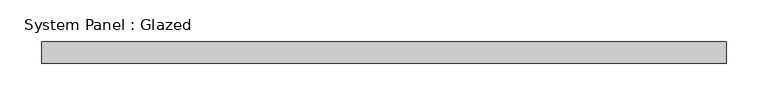
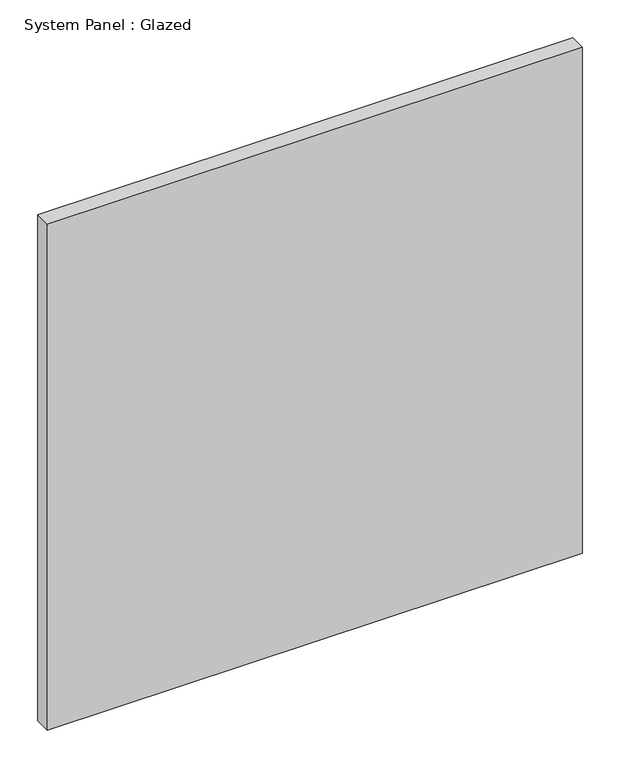
"""IFC4 building model written with IfcOpenShell, lengths in millimetres: plate geometry, System Panel : Glazed."""

from ifc_helpers import new_model, si_unit, origin, origin_with_axes, place, context, project, spatial, polyline, outline, extrude, source, transform, mapped, element, save


def system_panel_glazed_a79f7f85(model_context):
    return source(origin(), model_context, "Body", "SweptSolid", [
        extrude(outline(polyline([(409.575, 19.05), (-409.575, 19.05), (-409.575, 44.45), (409.575, 44.45), (409.575, 19.05)])), origin_with_axes(), (0.0, 0.0, 1.0), 819.15),
    ])


if __name__ == "__main__":
    model = new_model("IFC4")
    model_context = context("Model", 3, world=origin())
    ifc_project = project(units=[si_unit("LENGTHUNIT", "METRE", prefix="MILLI")], contexts=[model_context])
    site = spatial("IfcSite", under=ifc_project)
    building = spatial("IfcBuilding", under=site)
    placement = place(None, origin())
    system_panel_glazed_shape = system_panel_glazed_a79f7f85(model_context)
    element("IfcPlate", 1, ObjectType="System Panel : Glazed", at=placement, inside=building, context=model_context, shape_type="MappedRepresentation", body=[
        mapped(system_panel_glazed_shape, transform((0.0, 0.0, 0.0), x_axis=(1.0, 0.0, 0.0), y_axis=(0.0, 1.0, 0.0), z_axis=(0.0, 0.0, 1.0))),
    ])
    save(model, "model.ifc")

# Revit data of these elements
# Type "System Panel : Glazed"
#   Construction Type Id = "GSP4R"
#   Analytic Construction = "1/8 in Pilkington single glazing"
#   Visual Light Transmittance = 0.9
#   Solar Heat Gain Coefficient = 0.86
#   Heat Transfer Coefficient (U) = 6.7069 W/(m²·K)
# Element 1 (IfcPlate, "System Panel : Glazed")
#   Materials on its faces: "Glass"
# Materials
#   "Glass": class "Glass", colour RGB 0 128 192, transparency 0.75, Description = "Soda Lime Glass", Cost = 0
